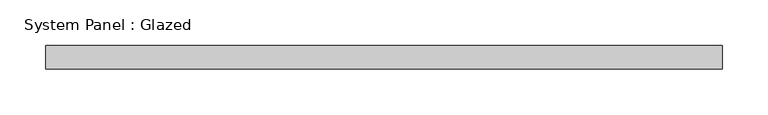
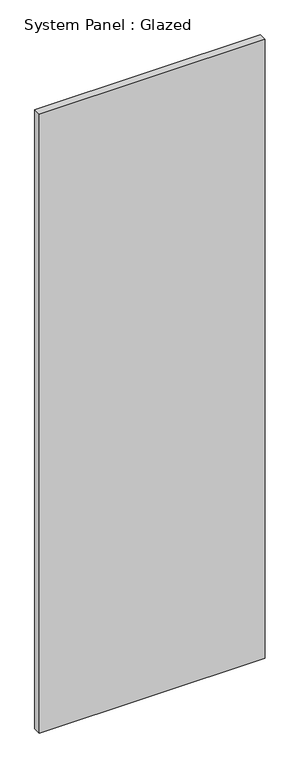
"""IFC4 building model written with IfcOpenShell, lengths in millimetres: plate geometry, System Panel : Glazed."""

from ifc_helpers import new_model, si_unit, origin, origin_with_axes, place, context, project, spatial, polyline, outline, extrude, source, transform, mapped, element, save


def system_panel_glazed_b407a8af(model_context):
    return source(origin(), model_context, "Body", "SweptSolid", [
        extrude(outline(polyline([(368.3, 19.05), (-368.3, 19.05), (-368.3, 44.45), (368.3, 44.45), (368.3, 19.05)])), origin_with_axes(), (0.0, 0.0, 1.0), 2133.6),
    ])


if __name__ == "__main__":
    model = new_model("IFC4")
    model_context = context("Model", 3, world=origin())
    ifc_project = project(units=[si_unit("LENGTHUNIT", "METRE", prefix="MILLI")], contexts=[model_context])
    site = spatial("IfcSite", under=ifc_project)
    building = spatial("IfcBuilding", under=site)
    placement = place(None, origin())
    system_panel_glazed_shape = system_panel_glazed_b407a8af(model_context)
    element("IfcPlate", 1, ObjectType="System Panel : Glazed", at=placement, inside=building, context=model_context, shape_type="MappedRepresentation", body=[
        mapped(system_panel_glazed_shape, transform((0.0, 0.0, 0.0), x_axis=(1.0, 0.0, 0.0), y_axis=(0.0, 1.0, 0.0), z_axis=(0.0, 0.0, 1.0))),
    ])
    save(model, "model.ifc")

# Revit data of these elements
# Type "System Panel : Glazed"
#   Construction Type Id = "GSP4R"
#   Analytic Construction = "1/8 in Pilkington single glazing"
#   Visual Light Transmittance = 0.9
#   Solar Heat Gain Coefficient = 0.86
#   Heat Transfer Coefficient (U) = 1.18115 BTU/(h·ft²·°F)
#   Define Thermal Properties by = 1
# Element 1 (IfcPlate, "System Panel : Glazed")
#   Materials on its faces: "Glass"
# Materials
#   "Glass": class "Glass", colour RGB 0 128 192, transparency 0.75, Description = "Soda Lime Glass", Cost = 0
